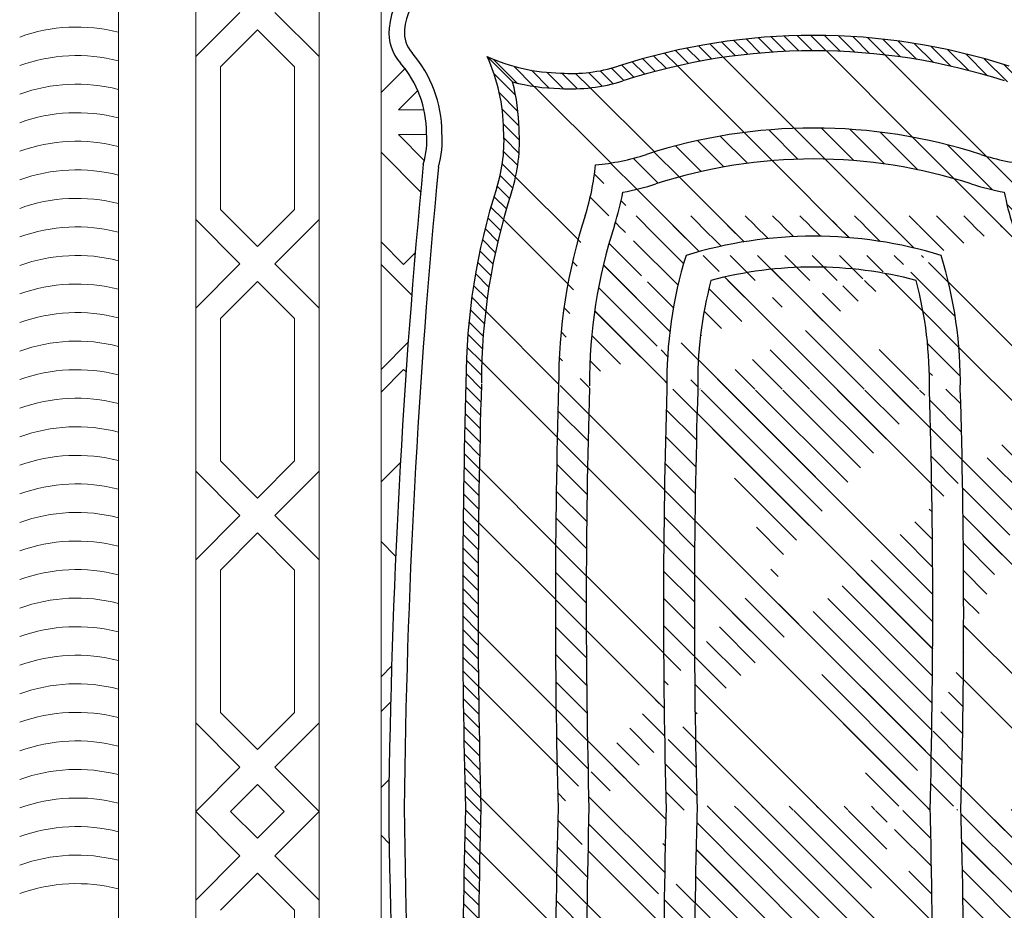
# Model space of a CAD drawing. Units: inches. Extents: x 3592 to 4861, y 1650 to 2243.
# Tile 8 of 30: x 4188.22 to 4207.34, y 1932.29 to 1949.57. Entities that reach past the tile are written whole.
import ezdxf

# ---------------------------------------------------------------- set-up
doc = ezdxf.new("R2010")
doc.units = ezdxf.units.IN
doc.layers.add('A-FURN', color=9, linetype='Continuous', lineweight=13)
doc.layers.add('RA-AP-01$0$INT', color=35, linetype='Continuous', lineweight=5)
for name, color, linetype in [('RA-AP-01$0$FURN', 3, 'Continuous'), ('RA-AP-01$0$WOOD', 64, 'Continuous'), ('RA-AP-02$0$FLPT', 30, 'Continuous')]:
    doc.layers.add(name, color=color, linetype=linetype)

# ---------------------------------------------------------------- blocks, each defined once
blk = doc.blocks.new('A$C67D63ADA')
at = {"layer": 'RA-AP-01$0$INT'}
for p, q in [((4.423181125509104, -6.89561531533655), (4.423181125509032, -6.912102561826093)), ((4.43918112550911, -6.893970246191535), (4.439181125509032, -6.912102561826071)), ((4.439181125509032, -6.912102561826071), (4.455879744655667, -6.89540394267944)), ((4.423181125509032, -6.912102561826093), (4.410714462739163, -6.899635899056222)), ((4.45049483400792, -6.923416270325152), (4.476136761728802, -6.897774342604276)), ((4.515810631825746, -6.901300610639258), (4.523298874513885, -6.908788853327399)), ((4.411867417009952, -6.923416270324986), (4.396098836558103, -6.907647689873135)), ((4.508671457515881, -6.923416270325402), (4.523298874513887, -6.908788853327399)), ((4.543172726542809, -6.903542418296127), (4.523298874513629, -6.923416270325749)), ((4.573619638989622, -6.905854783807836), (4.591181125507156, -6.923416270325372)), ((4.592759678002034, -6.907210300832407), (4.591181125507033, -6.908788853327405)), ((4.591181125507033, -6.908788853327405), (4.605808542505001, -6.923416270325372)), ((4.605808542505038, -6.923416270325409), (4.591181125507032, -6.908788853327405)), ((4.663985166013, -6.923416270325169), (4.651465045800739, -6.910896150112908)), ((4.702612583010966, -6.92341627032501), (4.712072573463438, -6.913956279872539)), ((4.790044040513182, -6.923416270324652), (4.783212045278532, -6.916584275090002)), ((4.806473209230177, -6.917218022043679), (4.812671457513205, -6.923416270326709)), ((4.856598418240554, -6.918206146064184), (4.861808542503289, -6.923416270326919)), ((4.897949975540099, -6.918137752297184), (4.892671457510363, -6.923416270326919)), ((4.877240000006827, -6.923416270326986), (4.277240000006364, -6.923416270324413)), ((4.508671457515881, -6.923416270325401), (4.45049483400792, -6.923416270325152)), ((4.591181125507156, -6.923416270325372), (4.523298874513629, -6.923416270325749)), ((4.605808542505038, -6.923416270325408), (4.663985166013, -6.923416270325169)), ((4.702612583010965, -6.923416270325013), (4.790044040513182, -6.923416270324652)), ((4.877240000006825, -6.923416270326986), (5.477240000007288, -6.923416270324413)), ((4.388754718631812, -6.963416270321417), (4.360068427135066, -6.99210256182739)), ((4.49421056275124, -6.963416270301053), (4.522896854257212, -6.992102561797802)), ((4.551583145753959, -6.963416270316853), (4.522896854257213, -6.992102561822827)), ((4.657038989877026, -6.963416270301689), (4.685725281382997, -6.992102561798438)), ((4.714411572888969, -6.963416270301689), (4.685725281382997, -6.992102561798438)), ((4.819867417008399, -6.963416270316511), (4.848553708505145, -6.992102561822482)), ((4.848553708505147, -6.992102561822486), (4.877240000011487, -6.963416270325371)), ((4.905926291508504, -6.992102561822486), (4.877240000002164, -6.963416270325371)), ((4.934612583005253, -6.963416270316511), (4.905926291508508, -6.992102561822482)), ((4.395382135640173, -6.979416270312523), (4.371382135635868, -7.003416270324554)), ((4.487583145750843, -6.979416270297111), (4.395382135640173, -6.979416270312523)), ((4.487583145750843, -6.979416270297111), (4.511583145760048, -7.003416270298604)), ((4.558210562750208, -6.979416270320077), (4.534210562758016, -7.003416270319991)), ((4.650411572883545, -6.979416270304665), (4.558210562750208, -6.979416270320077)), ((4.650411572883545, -6.979416270304665), (4.674411572885833, -7.00341627029924)), ((4.721038989886534, -6.979416270300584), (4.697038989880161, -7.00341627029924)), ((4.721038989886534, -6.979416270300584), (4.813240000007903, -6.979416270315998)), ((4.813240000007903, -6.979416270315486), (4.837240000004343, -7.003416270319647)), ((4.941240000005749, -6.979416270315486), (4.917240000009309, -7.003416270319647)), ((5.033441010127117, -6.979416270300584), (4.941240000005749, -6.979416270315998)), ((4.859867417002312, -7.003416270323289), (4.877240000006826, -6.986043687324361)), ((4.89461258301134, -7.003416270323289), (4.877240000006826, -6.986043687324361)), ((4.395382135631553, -7.027416270312525), (4.371382135635868, -7.003416270324554)), ((4.48758314576926, -7.027416270297113), (4.511583145760048, -7.003416270298604)), ((4.558210562765816, -7.027416270320077), (4.534210562758016, -7.003416270319991)), ((4.650411572888129, -7.027416270304664), (4.674411572885833, -7.00341627029924)), ((4.721038989873787, -7.027416270300586), (4.697038989880161, -7.00341627029924)), ((4.813240000000789, -7.027416270315487), (4.837240000004343, -7.003416270319647)), ((4.859867417002312, -7.003416270323289), (4.877240000001861, -7.020788853328426)), ((4.89461258301134, -7.003416270323289), (4.877240000011791, -7.020788853328426)), ((4.941240000012863, -7.027416270315487), (4.917240000009309, -7.003416270319647)), ((4.388754718643982, -7.043416270321417), (4.360068427138701, -7.014729978825361)), ((4.494210562764795, -7.043416270301053), (4.52289685426085, -7.01472997879577)), ((4.551583145766129, -7.043416270316853), (4.522896854260848, -7.014729978820797)), ((4.657038989890581, -7.043416270301689), (4.685725281386635, -7.014729978796407)), ((4.714411572875414, -7.043416270301689), (4.685725281379359, -7.014729978796407)), ((4.819867416996229, -7.04341627031651), (4.848553708501509, -7.014729978820453)), ((4.848553708501509, -7.014729978820453), (4.877239999998625, -7.043416270326798)), ((4.905926291512142, -7.014729978820453), (4.877240000015027, -7.043416270326798)), ((4.934612583017423, -7.04341627031651), (4.905926291512142, -7.014729978820453)), ((4.48758314576926, -7.027416270297113), (4.395382135631553, -7.027416270312525)), ((4.650411572888129, -7.027416270304664), (4.558210562765816, -7.027416270320077)), ((4.721038989873787, -7.027416270300586), (4.813239999999876, -7.027416270315999))]:
    blk.add_line(p, q, dxfattribs=at)
for points in [[(5.647240000006826, -6.243416270325369), (5.647240000006826, -7.09341627032537), (4.107240000006826, -7.093416270325372), (4.107240000006826, -6.19341627032537), (4.877240000006826, -6.19341627032537)], [(4.877240000006826, -6.19341627032537), (5.647240000006826, -6.19341627032537), (5.647240000006826, -7.09341627032537), (4.877240000006826, -7.09341627032537)], [(5.597240000006826, -6.243416270325369), (5.597240000006826, -7.04341627032537), (4.157240000006826, -7.043416270325372), (4.157240000006826, -6.243416270325369)], [(4.877240000006826, -6.32341627032537), (4.237240000006825, -6.32341627032537), (4.237240000006825, -6.963416270325371), (4.877240000006826, -6.963416270325371)], [(4.877240000006826, -6.32341627032537), (5.517240000006826, -6.32341627032537), (5.517240000006826, -6.963416270325371), (4.877240000006826, -6.963416270325371)]]:
    blk.add_lwpolyline(points, dxfattribs=at)
for centre, start in [((4.4787219589605, -7.120376270324156), 165.6974573648693), ((4.497201958964411, -7.120376270325429), 165.6974573641792), ((4.515681958963228, -7.120376270326884), 165.697457363391), ((4.534161958959862, -7.12037627032452), 165.697457364672), ((4.552641958963591, -7.120376270324702), 165.6974573645733), ((4.571121958962589, -7.120376270325975), 165.6974573638838), ((4.589601958963954, -7.120376270327248), 165.6974573631937), ((4.608081958962952, -7.120376270325065), 165.6974573643761), ((4.626561958964317, -7.120376270325248), 165.6974573642769), ((4.626561958963465, -7.120376270327612), 165.6974573629959), ((4.645041958962464, -7.120376270325429), 165.6974573641788), ((4.663521958961464, -7.120376270325429), 165.6974573641788), ((4.682001958965192, -7.120376270326703), 165.6974573634886), ((4.700481958964191, -7.120376270325794), 165.6974573639815), ((4.718961958960644, -7.120376270325794), 165.6974573639815), ((4.737441958964554, -7.120376270327067), 165.6974573632914), ((4.755921958963371, -7.120376270328522), 165.6974573625031), ((4.774401958960006, -7.120376270326158), 165.6974573637841), ((4.792881958963734, -7.120376270326339), 165.697457363686), ((4.811361958962733, -7.120376270327612), 165.6974573629959), ((4.829841958964097, -7.120376270328886), 165.6974573623059), ((4.848321958963096, -7.120376270326703), 165.6974573634886), ((4.86680195896446, -7.120376270326884), 165.6974573633905), ((4.885281958960913, -7.120376270329249), 165.6974573621089), ((4.903761958964823, -7.120376270329431), 165.6974573620104), ((4.92224195896364, -7.120376270327067), 165.6974573632914), ((4.940721958962639, -7.12037627032834), 165.6974573626018), ((4.959201958964003, -7.120376270329796), 165.6974573618131), ((4.977681958963002, -7.120376270329796), 165.6974573618131), ((4.996161958962002, -7.120376270327612), 165.6974573629959), ((5.014641958961001, -7.120376270327612), 165.6974573629959), ((5.033121958964729, -7.120376270328886), 165.6974573623059)]:
    blk.add_arc(centre, 0.1091312342836184, start, 199.7961568705686, dxfattribs=at)
blk = doc.blocks.new('A$C09A87C41')
at = {"layer": 'RA-AP-01$0$WOOD'}
h = blk.add_hatch(dxfattribs=at)
h.set_pattern_fill('ANSI31', color=256, scale=0.05, style=0)
h.set_pattern_definition([(45, (0.7182879904584168, -11.54818755465011), (0.0044194173824159, -0.0044194173824159), [])])
edge = h.paths.add_edge_path()
edge.add_ellipse((5.006516613079209, -11.27459283286495), major_axis=(3.435359877543153, 3.435359877543153), ratio=0.9999999999999982, start_angle=403.3022422558093, end_angle=406.5486575131389, ccw=False)
edge.add_ellipse((5.150455045735207, -6.828790194879051), major_axis=(-0.2901946312779826, 0.2901946312779826), ratio=0.9999999999999875, start_angle=297.2093186994243, end_angle=314.9999999999731, ccw=False)
edge.add_ellipse((5.307117976013378, -6.343033378039902), major_axis=(-0.0707106781186454, 0.0707106781186455), ratio=0.9999999999999651, start_angle=116.7779839927149, end_angle=139.0873288843009)
edge.add_ellipse((5.312718414970339, -6.324818905441738), major_axis=(0.0834173982641243, 0.0834173982641243), ratio=0.9999999999999847, start_angle=225.741775187377, end_angle=249.5633269497028)
edge.add_line((5.361758401537698, -6.432112914518591), (5.345299417747169, -6.448571898309089))
edge.add_ellipse((5.312718414970311, -6.32481890544173), major_axis=(-0.0904884660759946, 0.0904884660759945), ratio=0.9999999999999644, start_angle=135.8720682536374, end_angle=149.7498089726665, ccw=False)
edge.add_ellipse((5.307117976013483, -6.343033378039922), major_axis=(-0.0777817459304867, 0.0777817459304867), ratio=0.9999999999999941, start_angle=117.45144083316339, end_angle=138.9346900893823, ccw=False)
edge.add_ellipse((5.150455045735208, -6.82879019487905), major_axis=(0.2831235634661059, 0.2831235634661059), ratio=0.9999999999999859, start_angle=27.03507540014952, end_angle=44.9867285887044)
edge.add_ellipse((5.006516315412802, -11.27459997798134), major_axis=(-3.428298916554014, 3.428298916554014), ratio=0.9999999999999971, start_angle=-46.70235550375367, end_angle=-43.44815559494434)
edge.add_ellipse((4.743915471599394, -11.2745999779814), major_axis=(3.428298916553931, 3.42829891655393), ratio=0.9999999999999994, start_angle=43.44815559494427, end_angle=46.70235550375375)
edge.add_ellipse((4.599976741276995, -6.828790194879051), major_axis=(0.2831235634661173, 0.2831235634661172), ratio=0.9999999999999861, start_angle=45.01327141129749, end_angle=62.96492459984043)
edge.add_ellipse((4.443313810998718, -6.343033378039922), major_axis=(0.0777817459304893, 0.0777817459304893), ratio=0.9999999999999873, start_angle=221.0653099106178, end_angle=242.54855916687399, ccw=False)
edge.add_ellipse((4.437713372041892, -6.32481890544173), major_axis=(0.0904884660759951, 0.0904884660759951), ratio=0.9999999999999603, start_angle=210.2501910273332, end_angle=224.1279317463614, ccw=False)
edge.add_line((4.405132369265034, -6.448571898309089), (4.388673385474508, -6.432112914518594))
edge.add_ellipse((4.43771337204186, -6.324818905441737), major_axis=(0.0834173982641232, 0.0834173982641232), ratio=0.9999999999999797, start_angle=200.4366730503009, end_angle=224.2582248126243)
edge.add_ellipse((4.443313810998827, -6.343033378039902), major_axis=(-0.0707106781186382, 0.0707106781186382), ratio=0.9999999999999952, start_angle=130.9126711156974, end_angle=153.2220160072772)
edge.add_ellipse((4.599976741276995, -6.828790194879051), major_axis=(-0.2901946312779718, 0.2901946312779718), ratio=0.9999999999999895, start_angle=315.0000000000233, end_angle=332.7906813005773, ccw=False)
edge.add_ellipse((4.743915173933024, -11.27459283286497), major_axis=(-3.435359877543123, 3.435359877543123), ratio=0.9999999999999991, start_angle=313.451342486861, end_angle=316.69775774419077, ccw=False)
edge = h.paths.add_edge_path()
edge.add_ellipse((4.299593848995801, -6.48675334004306), major_axis=(-0.0707106781186556, 0.0707106781186556), ratio=0.9999999999999859, start_angle=206.7779839906583, end_angle=229.0873288838364)
edge.add_ellipse((4.281379376397651, -6.481152901086075), major_axis=(-0.0834173982641623, 0.0834173982641623), ratio=0.9999999999999754, start_angle=225.7417751869729, end_angle=249.5633269497573)
edge.add_line((4.388673385474506, -6.432112914518592), (4.405132369265034, -6.448571898309089))
edge.add_ellipse((4.281379376397657, -6.481152901086004), major_axis=(-0.0904884660760182, 0.0904884660760182), ratio=0.9999999999999957, start_angle=225.8720682533453, end_angle=239.7498089726896, ccw=False)
edge.add_ellipse((4.299593848995796, -6.486753340043026), major_axis=(0.0777817459305317, 0.0777817459305317), ratio=0.9999999999999891, start_angle=297.4514408381613, end_angle=318.9346900891407, ccw=False)
edge.add_ellipse((4.785350665835052, -6.643416270320893), major_axis=(0.2831235634661102, 0.2831235634661102), ratio=0.9999999999999978, start_angle=117.0350753988375, end_angle=152.9649246009711)
edge.add_ellipse((4.299593848995777, -6.800079200598784), major_axis=(-0.0777817459305426, 0.0777817459305426), ratio=0.9999999999999973, start_angle=221.0653099111909, end_angle=242.5485591625442, ccw=False)
edge.add_ellipse((4.281379376397679, -6.805679639555494), major_axis=(-0.0904884660760244, 0.0904884660760244), ratio=0.9999999999999076, start_angle=210.2501910270576, end_angle=224.1279317467988, ccw=False)
edge.add_line((4.405132369264926, -6.838260642332959), (4.388673385474263, -6.854719626123697))
edge.add_ellipse((4.281379376397679, -6.80567963955562), major_axis=(0.0834173982641642, 0.0834173982641642), ratio=0.9999999999999609, start_angle=290.4366730499258, end_angle=314.2582248131156)
edge.add_ellipse((4.299593848995804, -6.800079200598786), major_axis=(-0.0707106781186612, 0.0707106781186612), ratio=0.999999999999977, start_angle=220.9126711163551, end_angle=243.222016008517)
edge.add_ellipse((4.785350665835053, -6.643416270320894), major_axis=(0.2901946312779783, 0.2901946312779783), ratio=0.9999999999999984, start_angle=117.2093186999746, end_angle=152.7906813002342, ccw=False)
edge = h.paths.add_edge_path()
edge.add_ellipse((4.743915471599392, -2.012232562660299), major_axis=(3.428298916553894, 3.428298916553894), ratio=0.9999999999999992, start_angle=223.2976444962459, end_angle=226.5518444050561)
edge.add_ellipse((5.006516315412771, -2.012232562660296), major_axis=(3.428298916553752, 3.428298916553752), ratio=0.9999999999999971, start_angle=223.448155594945, end_angle=226.7023555037531)
edge.add_ellipse((5.150455045735209, -6.458042345762599), major_axis=(0.283123563466111, 0.283123563466111), ratio=0.999999999999996, start_angle=225.0132714112834, end_angle=242.9649246011241)
edge.add_ellipse((5.30711797601273, -6.94379916260194), major_axis=(0.0777817459305174, 0.0777817459305174), ratio=0.9999999999999873, start_angle=401.06530991071423, end_angle=422.548559161793, ccw=False)
edge.add_ellipse((5.312718414969516, -6.962013635200094), major_axis=(0.0904884660760023, 0.0904884660760023), ratio=0.9999999999999566, start_angle=390.2501910269164, end_angle=404.12793174642553, ccw=False)
edge.add_line((5.345299417747278, -6.838260642332959), (5.361758401537942, -6.854719626123698))
edge.add_ellipse((5.312718414969516, -6.962013635200098), major_axis=(0.0834173982641439, 0.0834173982641439), ratio=0.9999999999999785, start_angle=20.43667304973462, end_angle=44.25822481258737)
edge.add_ellipse((5.307117976012772, -6.943799162601948), major_axis=(-0.0707106781186618, 0.0707106781186618), ratio=0.999999999999977, start_angle=-49.08732888421749, end_angle=-26.77798399064677)
edge.add_ellipse((5.150455045735209, -6.458042345762597), major_axis=(0.2901946312779783, 0.2901946312779783), ratio=0.9999999999999957, start_angle=225.0000000000273, end_angle=242.7906812999824, ccw=False)
edge.add_ellipse((5.006516613079198, -2.012239707776725), major_axis=(3.43535987754352, 3.43535987754352), ratio=0.999999999999996, start_angle=223.4513424868609, end_angle=226.697757744191, ccw=False)
edge.add_ellipse((4.743915173933023, -2.012239707776712), major_axis=(3.435359877543229, 3.435359877543229), ratio=0.9999999999999998, start_angle=223.3022422558095, end_angle=226.5486575131387, ccw=False)
edge.add_ellipse((4.599976741276995, -6.458042345762597), major_axis=(0.2901946312779746, 0.2901946312779748), ratio=0.9999999999999964, start_angle=207.2093187000184, end_angle=224.9999999999795, ccw=False)
edge.add_ellipse((4.443313810999427, -6.943799162601947), major_axis=(-0.070710678118668, 0.070710678118668), ratio=0.9999999999999838, start_angle=-63.22201600935903, end_angle=-40.9126711157662)
edge.add_ellipse((4.437713372042683, -6.962013635200099), major_axis=(0.0834173982641484, 0.0834173982641484), ratio=0.9999999999999729, start_angle=45.74177518742643, end_angle=69.56332695026246)
edge.add_line((4.388673385474263, -6.854719626123697), (4.405132369264926, -6.838260642332958))
edge.add_ellipse((4.437713372042681, -6.962013635200094), major_axis=(0.0904884660760224, 0.0904884660760225), ratio=0.9999999999999282, start_angle=405.87206825357924, end_angle=419.7498089730807, ccw=False)
edge.add_ellipse((4.443313810999475, -6.94379916260194), major_axis=(-0.0777817459305165, 0.0777817459305165), ratio=0.9999999999999927, start_angle=297.4514408382556, end_angle=318.93469008929503, ccw=False)
edge.add_ellipse((4.599976741276995, -6.458042345762597), major_axis=(0.2831235634661077, 0.2831235634661077), ratio=0.9999999999999937, start_angle=207.0350753988627, end_angle=224.9867285886981)
edge = h.paths.add_edge_path()
edge.add_ellipse((5.450837938016399, -6.800079200598789), major_axis=(-0.0707106781186565, 0.0707106781186565), ratio=0.9999999999999875, start_angle=26.77798399147072, end_angle=49.08732888364846)
edge.add_ellipse((5.469052410614524, -6.80567963955562), major_axis=(0.0834173982641601, 0.0834173982641601), ratio=0.9999999999999984, start_angle=135.7417751868887, end_angle=159.563326950074)
edge.add_line((5.36175840153794, -6.854719626123697), (5.345299417747278, -6.838260642332959))
edge.add_ellipse((5.469052410614523, -6.805679639555488), major_axis=(0.0904884660760307, 0.0904884660760307), ratio=0.9999999999999984, start_angle=135.8720682531977, end_angle=149.7498089729454, ccw=False)
edge.add_ellipse((5.450837938016426, -6.800079200598787), major_axis=(0.0777817459305426, 0.0777817459305427), ratio=0.9999999999999968, start_angle=117.4514408374904, end_angle=138.9346900888003, ccw=False)
edge.add_ellipse((4.965081121177151, -6.643416270320895), major_axis=(-0.2831235634661119, 0.2831235634661119), ratio=0.9999999999999992, start_angle=207.0350753990193, end_angle=242.9649246011595)
edge.add_ellipse((5.450837938016407, -6.486753340043026), major_axis=(0.0777817459305285, 0.0777817459305285), ratio=0.9999999999999747, start_angle=131.0653099108597, end_angle=152.5485591618505, ccw=False)
edge.add_ellipse((5.469052410614547, -6.481152901086004), major_axis=(0.09048846607603, 0.09048846607603), ratio=0.9999999999999619, start_angle=120.25019102731059, end_angle=134.1279317466551, ccw=False)
edge.add_line((5.345299417747169, -6.448571898309089), (5.361758401537697, -6.432112914518592))
edge.add_ellipse((5.469052410614551, -6.481152901086075), major_axis=(-0.0834173982641603, 0.0834173982641603), ratio=0.9999999999999998, start_angle=20.43667305024269, end_angle=44.25822481302925)
edge.add_ellipse((5.450837938016403, -6.486753340043062), major_axis=(-0.0707106781186603, 0.0707106781186603), ratio=0.9999999999999737, start_angle=40.91267111616517, end_angle=63.22201600943157)
edge.add_ellipse((4.965081121177149, -6.643416270320895), major_axis=(0.2901946312779771, 0.2901946312779771), ratio=0.9999999999999992, start_angle=297.2093186997686, end_angle=332.7906813000034, ccw=False)
h = blk.add_hatch(dxfattribs=at)
h.set_pattern_fill('ANSI32', color=256, scale=0.2, style=0)
h.set_pattern_definition([(45, (0.7182879904584168, -11.54818755465011), (0.0530330085889911, -0.0530330085889911), []), (45, (0.7182879904584168, -11.51283221565011), (0.0530330085889911, -0.0530330085889911), [])])
edge = h.paths.add_edge_path()
edge.add_ellipse((5.15045504573521, -6.82879019487905), major_axis=(-0.2831235634661157, 0.2831235634661156), ratio=0.9999999999999889, start_angle=297.21454354460053, end_angle=314.98672858870884, ccw=False)
edge.add_ellipse((5.307117976013485, -6.343033378039922), major_axis=(-0.0777817459304881, 0.0777817459304881), ratio=0.9999999999999928, start_angle=116.7981781115797, end_angle=138.9346900893818)
edge.add_ellipse((5.312718414970311, -6.32481890544173), major_axis=(-0.0904884660759946, 0.0904884660759946), ratio=0.9999999999999658, start_angle=135.8720682536378, end_angle=149.7498089726664)
edge.add_ellipse((5.469052410614547, -6.481152901086004), major_axis=(0.0904884660760303, 0.0904884660760302), ratio=0.9999999999999603, start_angle=120.2501910273106, end_angle=134.1279317466551)
edge.add_ellipse((5.450837938016407, -6.486753340043026), major_axis=(-0.0777817459305327, 0.0777817459305327), ratio=0.9999999999999915, start_angle=41.06530991085969, end_angle=63.20182189333976)
edge.add_ellipse((4.965081121177151, -6.643416270320894), major_axis=(-0.2831235634661133, 0.2831235634661133), ratio=0.9999999999999984, start_angle=207.214543545815, end_angle=242.7854564539869, ccw=False)
edge.add_ellipse((5.450837938016426, -6.800079200598786), major_axis=(0.0777817459305424, 0.0777817459305424), ratio=0.9999999999999962, start_angle=116.7981781073729, end_angle=138.9346900888086)
edge.add_ellipse((5.469052410614524, -6.805679639555493), major_axis=(0.0904884660760289, 0.0904884660760289), ratio=0.9999999999999841, start_angle=135.872068253202, end_angle=149.7498089729424)
edge.add_ellipse((5.312718414969522, -6.962013635200094), major_axis=(-0.0904884660760224, 0.0904884660760225), ratio=0.9999999999999282, start_angle=-59.7498089730807, end_angle=-45.87206825357926)
edge.add_ellipse((5.307117976012728, -6.94379916260194), major_axis=(0.0777817459305181, 0.0777817459305181), ratio=0.9999999999999861, start_angle=41.06530991070497, end_angle=63.20182189334603)
edge.add_ellipse((5.150455045735208, -6.458042345762599), major_axis=(0.2831235634661146, 0.2831235634661146), ratio=0.9999999999999907, start_angle=225.013271411291, end_angle=242.7854564539341, ccw=False)
edge.add_ellipse((5.006516315412806, -2.012232562660296), major_axis=(3.428298916554143, 3.428298916554143), ratio=0.9999999999999941, start_angle=223.4481555949448, end_angle=226.7023555037533, ccw=False)
edge.add_ellipse((4.743915471599424, -2.012232562660299), major_axis=(3.428298916554168, 3.428298916554171), ratio=0.9999999999999991, start_angle=223.2976444962462, end_angle=226.551844405056, ccw=False)
edge.add_ellipse((4.599976741276996, -6.458042345762597), major_axis=(0.2831235634661098, 0.2831235634661098), ratio=0.9999999999999973, start_angle=207.2145435460398, end_angle=224.9867285887048, ccw=False)
edge.add_ellipse((4.443313810999473, -6.94379916260194), major_axis=(-0.0777817459305183, 0.0777817459305183), ratio=0.9999999999999823, start_angle=-63.2018218932521, end_angle=-41.06530991071377)
edge.add_ellipse((4.437713372042686, -6.962013635200094), major_axis=(-0.0904884660760028, 0.0904884660760028), ratio=0.9999999999999504, start_angle=-44.12793174642511, end_angle=-30.25019102691602)
edge.add_ellipse((4.281379376397679, -6.80567963955549), major_axis=(-0.0904884660760215, 0.0904884660760215), ratio=0.9999999999999245, start_angle=210.2501910270558, end_angle=224.1279317467963)
edge.add_ellipse((4.299593848995777, -6.800079200598786), major_axis=(0.077781745930539, 0.077781745930539), ratio=0.999999999999963, start_angle=311.0653099111909, end_angle=333.2018218926339)
edge.add_ellipse((4.785350665835052, -6.643416270320894), major_axis=(0.2831235634661089, 0.2831235634661091), ratio=0.9999999999999989, start_angle=117.21454354600829, end_angle=152.7854564541833, ccw=False)
edge.add_ellipse((4.299593848995796, -6.486753340043026), major_axis=(0.077781745930533, 0.077781745930533), ratio=0.9999999999999792, start_angle=296.7981781066777, end_angle=318.9346900891398)
edge.add_ellipse((4.281379376397657, -6.481152901086003), major_axis=(-0.0904884660760217, 0.0904884660760217), ratio=0.9999999999999742, start_angle=225.872068253344, end_angle=239.7498089726891)
edge.add_ellipse((4.437713372041892, -6.32481890544173), major_axis=(0.090488466075997, 0.090488466075997), ratio=0.9999999999999756, start_angle=210.2501910273331, end_angle=224.1279317463622)
edge.add_ellipse((4.44331381099872, -6.343033378039923), major_axis=(0.0777817459304873, 0.0777817459304872), ratio=0.9999999999999861, start_angle=221.0653099106177, end_angle=243.2018218883976)
edge.add_ellipse((4.599976741276995, -6.828790194879051), major_axis=(-0.2831235634661067, 0.2831235634661067), ratio=0.9999999999999895, start_angle=315.01327141129775, end_angle=332.78545645540567, ccw=False)
edge.add_ellipse((4.743915471599392, -11.2745999779814), major_axis=(-3.428298916553902, 3.428298916553902), ratio=0.9999999999999984, start_angle=313.4481555949443, end_angle=316.7023555037538, ccw=False)
edge.add_ellipse((5.006516315412786, -11.27459997798134), major_axis=(-3.428298916554052, 3.428298916554052), ratio=1, start_angle=313.29764449624645, end_angle=316.5518444050555, ccw=False)
edge = h.paths.add_edge_path(flags=16)
edge.add_ellipse((4.745320840887742, -11.27459782170807), major_axis=(3.392940520945516, 3.392940520945516), ratio=1, start_angle=43.44876692339471, end_angle=46.71249975461917)
edge.add_ellipse((4.599976741276995, -6.828790194878992), major_axis=(-0.2477682244067734, 0.2477682244067734), ratio=0.9999999999999911, start_angle=-45.31868720933983, end_angle=-27.00912183057358)
edge.add_ellipse((4.443313810998828, -6.343033378039872), major_axis=(0.1131370849898469, 0.1131370849898469), ratio=0.9999999999999724, start_angle=230.5682590208478, end_angle=242.6218359751805, ccw=False)
edge.add_ellipse((4.299593848995757, -6.486753340043112), major_axis=(-0.1131370849898624, 0.1131370849898624), ratio=0.9999999999999953, start_angle=207.3781640250758, end_angle=219.4317409792351, ccw=False)
edge.add_ellipse((4.78535066583505, -6.643416270320884), major_axis=(0.2477682244067863, 0.2477682244067863), ratio=0.9999999999999974, start_angle=117.0091218305267, end_angle=152.9908781690427)
edge.add_ellipse((4.299593848995773, -6.800079200598856), major_axis=(0.1131370849898833, 0.1131370849898833), ratio=0.9999999999999682, start_angle=320.56825902084296, end_angle=332.62183597593753, ccw=False)
edge.add_ellipse((4.443313810999473, -6.943799162601939), major_axis=(0.1131370849898351, 0.1131370849898351), ratio=0.9999999999999213, start_angle=387.3781640246361, end_angle=399.43174097937606, ccw=False)
edge.add_ellipse((4.599976741276996, -6.458042345762606), major_axis=(0.2477682244067743, 0.2477682244067742), ratio=0.99999999999999, start_angle=207.0091218307682, end_angle=225.3186872093523)
edge.add_ellipse((4.745320840887777, -2.012234718933553), major_axis=(-3.392940520945741, 3.392940520945741), ratio=0.9999999999999992, start_angle=133.2875002453813, end_angle=136.5512330766047)
edge.add_ellipse((5.005110946124445, -2.012234718933546), major_axis=(3.392940520945412, 3.392940520945411), ratio=0.9999999999999989, start_angle=223.4487669233947, end_angle=226.7124997546191)
edge.add_ellipse((5.150455045735207, -6.458042345762608), major_axis=(-0.2477682244067739, 0.2477682244067739), ratio=0.9999999999999966, start_angle=134.6813127906568, end_angle=152.9908781692236)
edge.add_ellipse((5.30711797601273, -6.943799162601939), major_axis=(-0.1131370849898406, 0.1131370849898406), ratio=0.9999999999999811, start_angle=320.568259020624, end_angle=332.62183597538194, ccw=False)
edge.add_ellipse((5.45083793801643, -6.800079200598855), major_axis=(0.113137084989895, 0.113137084989895), ratio=0.999999999999955, start_angle=117.3781640240419, end_angle=129.4317409791577, ccw=False)
edge.add_ellipse((4.965081121177152, -6.643416270320884), major_axis=(0.2477682244067847, 0.2477682244067847), ratio=0.9999999999999992, start_angle=297.0091218309669, end_angle=332.990878169475)
edge.add_ellipse((5.450837938016447, -6.486753340043118), major_axis=(-0.1131370849898789, 0.1131370849898789), ratio=0.9999999999999342, start_angle=50.56825902076281, end_angle=62.62183597491821, ccw=False)
edge.add_ellipse((5.30711797601337, -6.34303337803987), major_axis=(0.1131370849898374, 0.1131370849898374), ratio=0.9999999999999493, start_angle=207.3781640247929, end_angle=219.4317409791543, ccw=False)
edge.add_ellipse((5.150455045735204, -6.828790194878992), major_axis=(-0.2477682244067807, 0.2477682244067808), ratio=0.9999999999999934, start_angle=-62.99087816941401, end_angle=-44.68131279065508)
edge.add_ellipse((5.005110946124442, -11.27459782170805), major_axis=(3.392940520945543, 3.392940520945543), ratio=0.9999999999999974, start_angle=43.28750024538099, end_angle=46.55123307660507)
edge = h.paths.add_edge_path(flags=0)
edge.add_ellipse((4.745321446260899, -11.27461227828643), major_axis=(3.378818834290158, 3.378818834290157), ratio=0.9999999999999996, start_angle=43.44228925150885, end_angle=46.72161971502517)
edge.add_ellipse((4.599976741276998, -6.828790194878991), major_axis=(-0.2336260887830454, 0.2336260887830454), ratio=0.9999999999999974, start_angle=-45.30974264369766, end_angle=-26.99844483641433)
edge.add_ellipse((4.443313810998811, -6.343033378039858), major_axis=(0.1272792206135962, 0.1272792206135962), ratio=0.9999999999999403, start_angle=235.6264990356023, end_angle=242.6432427499436, ccw=False)
edge.add_ellipse((4.299593848995773, -6.486753340043007), major_axis=(0.1272792206136285, 0.1272792206136286), ratio=0.9999999999999204, start_angle=297.35675724967757, end_angle=304.3735009644582, ccw=False)
edge.add_ellipse((4.785350665835048, -6.643416270320905), major_axis=(0.2336260887830504, 0.2336260887830504), ratio=0.9999999999999921, start_angle=116.998444836676, end_angle=153.0015551636886)
edge.add_ellipse((4.299593848995741, -6.800079200598703), major_axis=(-0.1272792206136906, 0.1272792206136906), ratio=0.9999999999996289, start_angle=235.62649903554922, end_angle=242.64324274961962, ccw=False)
edge.add_ellipse((4.443313810999469, -6.943799162601998), major_axis=(-0.1272792206136219, 0.1272792206136219), ratio=0.9999999999999658, start_angle=297.3567572500489, end_angle=304.3735009646209, ccw=False)
edge.add_ellipse((4.599976741276995, -6.458042345762605), major_axis=(0.2336260887830445, 0.2336260887830445), ratio=0.9999999999999957, start_angle=206.9984448365414, end_angle=225.3097426436968)
edge.add_ellipse((4.745321446260921, -2.012220262355212), major_axis=(3.378818834290089, 3.378818834290088), ratio=0.9999999999999994, start_angle=223.2783802849744, end_angle=226.5577107484907)
edge.add_ellipse((5.005110340751275, -2.012220262355198), major_axis=(3.378818834290274, 3.378818834290274), ratio=0.9999999999999992, start_angle=223.4422892515091, end_angle=226.7216197150253)
edge.add_ellipse((5.150455045735206, -6.458042345762609), major_axis=(0.2336260887830463, 0.2336260887830463), ratio=0.9999999999999937, start_angle=224.6902573562994, end_angle=243.0015551634542)
edge.add_ellipse((5.30711797601273, -6.943799162602), major_axis=(-0.1272792206135949, 0.1272792206135949), ratio=0.9999999999997138, start_angle=325.62649903537766, end_angle=332.6432427499585, ccw=False)
edge.add_ellipse((5.450837938016461, -6.800079200598699), major_axis=(-0.1272792206135936, 0.1272792206135936), ratio=0.999999999999666, start_angle=27.356757250387716, end_angle=34.37350096445232, ccw=False)
edge.add_ellipse((4.965081121177155, -6.643416270320904), major_axis=(0.23362608878305, 0.23362608878305), ratio=0.9999999999999992, start_angle=296.9984448363078, end_angle=333.0015551633219)
edge.add_ellipse((5.450837938016428, -6.486753340043003), major_axis=(0.1272792206136045, 0.1272792206136045), ratio=0.9999999999999529, start_angle=145.6264990355431, end_angle=152.6432427503271, ccw=False)
edge.add_ellipse((5.307117976013396, -6.34303337803986), major_axis=(0.1272792206135615, 0.1272792206135615), ratio=0.9999999999996925, start_angle=207.3567572500474, end_angle=214.3735009643965, ccw=False)
edge.add_ellipse((5.150455045735208, -6.828790194878991), major_axis=(-0.2336260887830484, 0.2336260887830485), ratio=0.9999999999999953, start_angle=-63.00155516358085, end_angle=-44.69025735630093)
edge.add_ellipse((5.005110340751286, -11.27461227828636), major_axis=(-3.378818834290266, 3.378818834290266), ratio=0.9999999999999998, start_angle=-46.72161971502535, end_angle=-43.44228925150914)
edge = h.paths.add_edge_path(flags=0)
edge.add_ellipse((4.747128261062206, -11.27459926241731), major_axis=(-3.343445075648777, 3.343445075648777), ratio=0.9999999999999991, start_angle=-46.55229325491085, end_angle=-43.26504392007965)
edge.add_ellipse((4.599976741277094, -6.828790194878977), major_axis=(0.198270749723715, 0.198270749723715), ratio=0.999999999999988, start_angle=44.18347671010175, end_angle=62.12936993332099)
edge.add_ellipse((4.785350665835048, -6.643416270320889), major_axis=(0.198270749723727, 0.198270749723727), ratio=0.9999999999999971, start_angle=117.8706300667295, end_angle=152.1293699332338)
edge.add_ellipse((4.599976741276998, -6.458042345762598), major_axis=(0.1982707497237202, 0.1982707497237202), ratio=0.9999999999999882, start_angle=207.8706300666892, end_angle=225.8165232899116)
edge.add_ellipse((4.747128261062279, -2.01223327822427), major_axis=(-3.343445075648579, 3.34344507564858), ratio=0.9999999999999984, start_angle=133.2650439200784, end_angle=136.5522932549098)
edge.add_ellipse((5.003303525949927, -2.012233278224277), major_axis=(-3.343445075648679, 3.343445075648679), ratio=0.9999999999999996, start_angle=133.4477067450899, end_angle=136.7349560799216)
edge.add_ellipse((5.150455045735204, -6.458042345762598), major_axis=(-0.1982707497237223, 0.1982707497237223), ratio=0.9999999999999994, start_angle=134.1834767100914, end_angle=152.1293699333112)
edge.add_ellipse((4.965081121177155, -6.643416270320892), major_axis=(0.1982707497237268, 0.1982707497237267), ratio=0.9999999999999987, start_angle=297.8706300667671, end_angle=332.1293699332712)
edge.add_ellipse((5.150455045735109, -6.828790194878977), major_axis=(0.1982707497237106, 0.1982707497237105), ratio=0.9999999999999982, start_angle=27.87063006667902, end_angle=45.8165232898948)
edge.add_ellipse((5.00330352595001, -11.2745992624173), major_axis=(3.343445075648743, 3.343445075648743), ratio=0.9999999999999996, start_angle=43.26504392007961, end_angle=46.55229325491089)
edge = h.paths.add_edge_path(flags=0)
edge.add_ellipse((4.747685770081003, -11.27459857725902), major_axis=(3.329301968186143, 3.329301968186141), ratio=0.9999999999999989, start_angle=43.44789769190167, end_angle=46.74269456932172)
edge.add_ellipse((4.599976741277087, -6.828790194878972), major_axis=(-0.1841286140999701, 0.1841286140999702), ratio=0.9999999999999841, start_angle=-45.99531238101485, end_angle=-30.22398030679106)
edge.add_ellipse((4.785350665835029, -6.643416270320906), major_axis=(0.1841286140999794, 0.1841286140999793), ratio=0.9999999999999998, start_angle=120.2239803068321, end_angle=149.7760196931203)
edge.add_ellipse((4.599976741276998, -6.458042345762589), major_axis=(0.1841286140999956, 0.1841286140999956), ratio=0.9999999999999953, start_angle=210.2239803068005, end_angle=225.9953123810239)
edge.add_ellipse((4.747685770081015, -2.012233963382593), major_axis=(-3.329301968186209, 3.32930196818621), ratio=0.9999999999999991, start_angle=133.2573054306775, end_angle=136.5521023080975)
edge.add_ellipse((5.002746016931159, -2.012233963382618), major_axis=(-3.329301968186245, 3.329301968186245), ratio=0.9999999999999984, start_angle=133.447897691902, end_angle=136.7426945693227)
edge.add_ellipse((5.150455045735208, -6.458042345762592), major_axis=(-0.1841286140999912, 0.1841286140999912), ratio=0.9999999999999873, start_angle=134.0046876189747, end_angle=149.7760196931988)
edge.add_ellipse((4.965081121177172, -6.643416270320907), major_axis=(-0.1841286140999788, 0.1841286140999788), ratio=0.9999999999999968, start_angle=210.2239803068796, end_angle=239.7760196931682)
edge.add_ellipse((5.150455045735117, -6.82879019487897), major_axis=(0.1841286140999714, 0.1841286140999713), ratio=0.9999999999999896, start_angle=30.22398030679139, end_angle=45.99531238102014)
edge.add_ellipse((5.002746016931209, -11.274598577259), major_axis=(3.329301968186158, 3.329301968186158), ratio=1, start_angle=43.25730543067866, end_angle=46.5521023080979)
h = blk.add_hatch(dxfattribs=at)
h.set_pattern_fill('ANSI31', color=256, scale=0.1, style=0)
h.set_pattern_definition([(45, (0.7182879904584168, -11.54818755465011), (0.0088388347648318, -0.0088388347648318), [])])
edge = h.paths.add_edge_path(flags=16)
edge.add_arc((4.965081121177173, -6.643416270320907), 0.2603971832811541, 345.2239803068796, 374.7760196931681)
edge.add_arc((4.965081121177173, -6.643416270320907), 0.2603971832811541, -14.776019693120418, 14.77601969316811, ccw=False)
edge = h.paths.add_edge_path(flags=16)
edge.add_arc((4.785350665835029, -6.643416270320907), 0.2603971832811541, 165.223980306832, 194.7760196931204)
edge.add_arc((4.785350665835029, -6.643416270320907), 0.2603971832811541, 165.223980306832, 194.7760196931204, ccw=False)
edge = h.paths.add_edge_path(flags=0)
edge.add_arc((4.785350665835029, -6.643416270320907), 0.2603971832811541, 165.223980306832, 194.7760196931204)
edge.add_arc((4.785350665835029, -6.643416270320907), 0.2603971832811541, 165.223980306832, 194.7760196931204, ccw=False)
edge = h.paths.add_edge_path(flags=0)
edge.add_arc((4.785350665835029, -6.643416270320907), 0.2603971832811541, 165.223980306832, 194.7760196931204)
edge.add_arc((4.785350665835029, -6.643416270320907), 0.2603971832811541, 165.223980306832, 194.7760196931204, ccw=False)
edge = h.paths.add_edge_path(flags=0)
edge.add_arc((4.785350665835029, -6.643416270320907), 0.2603971832811541, 165.223980306832, 194.7760196931204)
edge.add_arc((4.785350665835029, -6.643416270320907), 0.2603971832811541, 165.223980306832, 194.7760196931204, ccw=False)
edge = h.paths.add_edge_path(flags=0)
edge.add_arc((4.785350665835029, -6.643416270320907), 0.2603971832811541, 165.223980306832, 194.7760196931204)
edge.add_arc((4.785350665835029, -6.643416270320907), 0.2603971832811541, 165.223980306832, 194.7760196931204, ccw=False)
edge = h.paths.add_edge_path(flags=0)
edge.add_arc((4.785350665835029, -6.643416270320907), 0.2603971832811541, 165.223980306832, 194.7760196931204)
edge.add_arc((4.785350665835029, -6.643416270320907), 0.2603971832811541, 165.223980306832, 194.7760196931204, ccw=False)
edge = h.paths.add_edge_path(flags=0)
edge.add_arc((4.785350665835029, -6.643416270320907), 0.2603971832811541, 165.223980306832, 194.7760196931204)
edge.add_arc((4.785350665835029, -6.643416270320907), 0.2603971832811541, 165.223980306832, 194.7760196931204, ccw=False)
edge = h.paths.add_edge_path()
edge.add_arc((5.30711797601273, -6.943799162601939), 0.1599999999999918, 95.56825902062381, 107.6218359753744)
edge.add_arc((5.150455045735207, -6.458042345762605), 0.3503971832811637, 269.6813127906517, 287.9908781692269)
edge.add_arc((5.307117976013371, -6.34303337803987), 0.1599999999999917, 252.3781640232651, 264.4317409791539)
edge.add_arc((4.965081121177153, -6.643416270320884), 0.3503971832811761, 342.0091218309644, 377.9908781694648)
edge.add_arc((5.005110946124438, -2.012234718933557), 4.798342501046485, 268.4423197280547, 271.7124997546188)
edge.add_arc((5.150455045735207, -6.828790194878991), 0.3503971832811637, 72.00912183077308, 90.31868720934834)
edge.add_arc((5.005110340751293, -2.012220262355208), 4.778371420254705, 268.433225420277, 271.7034061068158)
edge.add_arc((5.150455045735207, -6.828790194878991), 0.3303971832811637, 72.00912183077308, 90.31868720934834)
edge.add_arc((5.005110340751291, -11.27461227828638), 4.7783714202547, 88.29659389318418, 91.5667745797229)
edge.add_arc((5.450837938016446, -6.486753340043115), 0.1600000000000254, 185.5682590207637, 197.6218359749416)
edge.add_arc((5.450837938016429, -6.800079200598855), 0.1600000000000541, 162.3781640240467, 174.4317409791574)
edge.add_arc((5.307117976012735, -6.943799162601998), 0.1800000000000505, 100.6264990353792, 107.6432427499818)
edge.add_arc((5.307117976013394, -6.343033378039859), 0.1800000000000069, 252.3567572486067, 259.3735009643972)
edge.add_arc((5.45083793801643, -6.486753340043007), 0.1800000000000424, 190.6264990355417, 197.6432427503393)
edge.add_arc((4.965081121177155, -6.643416270320905), 0.3303971832811676, 341.9984448362978, 378.0015551633146)
edge.add_arc((5.450837938016462, -6.800079200598699), 0.1800000000000547, 162.3567572504062, 169.373500964452)
edge.add_arc((5.150455045735206, -6.458042345762599), 0.2803971832811691, 269.1834767100981, 287.1293699333106)
edge.add_arc((5.150455045735107, -6.828790194878977), 0.2803971832811534, 72.87063006667864, 90.81652328989695)
edge.add_arc((4.965081121177155, -6.643416270320891), 0.2803971832811769, 342.8706300667665, 377.1293699332709)
edge.add_arc((5.150455045735205, -6.45804234576259), 0.2603971832811776, 269.0046876189688, 284.7760196931993)
edge.add_arc((5.150455045735117, -6.828790194878972), 0.2603971832811458, 75.22398030679119, 90.99531238102313)
edge.add_arc((5.150455045735207, -6.458042345762605), 0.3303971832811637, 269.6813127906517, 287.9908781692269)
edge.add_arc((5.003303525949946, -2.012233278224274), 4.728345371032053, 268.4320043718199, 271.7349560799219)
edge.add_arc((5.003303525949998, -11.27459926241731), 4.728345371032045, 88.2650439200796, 91.56799562818075)
edge.add_arc((5.00274601693117, -2.012233963382607), 4.708343996644348, 268.4295004240392, 271.7426945693223)
edge.add_arc((5.002746016931202, -11.274598577259), 4.708343996644358, 88.25730543067873, 91.57049957596126)
edge.add_arc((4.747685770080999, -11.274598577259), 4.708343996644359, 88.42950042403872, 91.74269456932127)
edge.add_arc((4.747685770081036, -2.012233963382596), 4.708343996644359, 268.2573054306777, 271.5704995759608)
edge.add_arc((4.747128261062202, -11.27459926241732), 4.728345371032054, 88.43200437181925, 91.73495607992041)
edge.add_arc((4.747128261062259, -2.012233278224274), 4.728345371032054, 268.265043920078, 271.56799562818)
edge.add_arc((4.74532144626091, -11.27461227828638), 4.778371420254699, 88.43322542027705, 91.7034061068158)
edge.add_arc((4.599976741276996, -6.828790194878991), 0.3303971832811637, 89.68131279065165, 107.9908781692269)
edge.add_arc((4.599976741276996, -6.458042345762605), 0.3303971832811637, 252.0091218307731, 270.3186872093484)
edge.add_arc((4.745321446260912, -2.012220262355208), 4.778371420254705, 268.2965938931842, 271.5667745797229)
edge.add_arc((4.599976741276996, -6.828790194878991), 0.3503971832811637, 89.68131279065165, 107.9908781692269)
edge.add_arc((4.745320840887767, -2.012234718933562), 4.79834250104648, 268.2875002453812, 271.5576802719454)
edge.add_arc((4.599976741277086, -6.828790194878972), 0.2603971832811458, 89.00468761897682, 104.7760196932087)
edge.add_arc((4.599976741276998, -6.45804234576259), 0.2603971832811776, 255.2239803068007, 270.9953123810312)
edge.add_arc((4.785350665835048, -6.643416270320891), 0.2803971832811769, 162.8706300667291, 197.1293699332334)
edge.add_arc((4.599976741277096, -6.828790194878977), 0.2803971832811534, 89.183476710103, 107.1293699333213)
edge.add_arc((4.599976741276996, -6.458042345762599), 0.2803971832811691, 252.8706300666894, 270.816523289902)
edge.add_arc((4.299593848995741, -6.800079200598699), 0.1800000000000547, 10.626499035548, 17.64324274959381)
edge.add_arc((4.785350665835048, -6.643416270320905), 0.3303971832811676, 161.9984448366853, 198.0015551637021)
edge.add_arc((4.299593848995773, -6.486753340043007), 0.1800000000000424, 342.3567572496606, 349.3735009644582)
edge.add_arc((4.44331381099881, -6.343033378039859), 0.1800000000000069, 280.6264990356027, 287.6432427513933)
edge.add_arc((4.443313810999468, -6.943799162601998), 0.1800000000000505, 72.35675725001818, 79.37350096462075)
edge.add_arc((4.299593848995773, -6.800079200598855), 0.1600000000000541, 5.568259020842612, 17.62183597595322)
edge.add_arc((4.78535066583505, -6.643416270320884), 0.3503971832811761, 162.0091218305351, 197.9908781690354)
edge.add_arc((4.299593848995757, -6.486753340043115), 0.1600000000000254, 342.3781640250583, 354.4317409792362)
edge.add_arc((4.443313810998832, -6.34303337803987), 0.1599999999999917, 275.5682590208461, 287.6218359767349)
edge.add_arc((4.599976741276996, -6.458042345762605), 0.3503971832811637, 252.0091218307731, 270.3186872093484)
edge.add_arc((4.443313810999473, -6.943799162601939), 0.1599999999999918, 72.37816402462555, 84.43174097937616)
edge.add_arc((5.005110946124436, -11.27459782170804), 4.798342501046482, 88.28750024538114, 91.55768027194539)
edge.add_arc((4.745320840887765, -11.27459782170804), 4.798342501046489, 88.44231972805461, 91.7124997546188)
blk.add_line((4.405132369264925, -6.838260642332959), (4.388673385474263, -6.854719626123697), dxfattribs=at)
blk.add_line((4.405132369264925, -6.838260642332959), (4.388673385474263, -6.854719626123697), dxfattribs=at)
for centre, radius, start, end in [((4.299593848995757, -6.486753340043115), 0.1600000000000254, 342.3781640250583, 354.4317409792362), ((4.785350665835053, -6.643416270320894), 0.4103971832811756, 162.0403002448635, 197.9596997549356), ((4.785350665835052, -6.643416270320894), 0.4003971832811741, 162.0350753988365, 197.9649246009689), ((4.299593848995773, -6.486753340043007), 0.1800000000000424, 342.3567572496606, 349.3735009644582), ((4.44331381099881, -6.343033378039859), 0.1800000000000069, 280.6264990356027, 287.6432427513933), ((4.78535066583505, -6.643416270320884), 0.3503971832811761, 162.0091218305351, 197.9908781690354), ((4.785350665835048, -6.643416270320905), 0.3303971832811676, 161.9984448366853, 198.0015551637021), ((4.599976741277096, -6.828790194878977), 0.2803971832811534, 89.183476710103, 107.1293699333213), ((4.747128261062202, -11.27459926241732), 4.728345371032054, 88.43200437181925, 91.73495607992041), ((5.003303525949998, -11.27459926241731), 4.728345371032045, 88.2650439200796, 91.56799562818075), ((4.785350665835048, -6.643416270320891), 0.2803971832811769, 162.8706300667291, 197.1293699332334), ((4.599976741277086, -6.828790194878972), 0.2603971832811458, 89.00468761897682, 104.7760196932087), ((4.747685770080999, -11.274598577259), 4.708343996644359, 88.42950042403872, 91.74269456932127), ((5.002746016931202, -11.274598577259), 4.708343996644358, 88.25730543067873, 91.57049957596126), ((4.785350665835029, -6.643416270320907), 0.2603971832811541, 165.223980306832, 194.7760196931204), ((4.785350665835029, -6.643416270320907), 0.2603971832811541, 165.223980306832, 194.7760196931204), ((4.599976741276998, -6.45804234576259), 0.2603971832811776, 255.2239803068007, 270.9953123810312), ((4.747685770081036, -2.012233963382596), 4.708343996644359, 268.2573054306777, 271.5704995759608), ((5.00274601693117, -2.012233963382607), 4.708343996644348, 268.4295004240392, 271.7426945693223), ((4.599976741276996, -6.458042345762599), 0.2803971832811691, 252.8706300666894, 270.816523289902), ((4.747128261062259, -2.012233278224274), 4.728345371032054, 268.265043920078, 271.56799562818), ((5.003303525949946, -2.012233278224274), 4.728345371032053, 268.4320043718199, 271.7349560799219), ((4.299593848995741, -6.800079200598699), 0.1800000000000547, 10.626499035548, 17.64324274959381), ((4.299593848995773, -6.800079200598855), 0.1600000000000541, 5.568259020842612, 17.62183597595322), ((4.299593848995777, -6.800079200598786), 0.1100000000000303, 356.0653099111937, 17.54855916255237), ((4.443313810999468, -6.943799162601998), 0.1800000000000505, 72.35675725001818, 79.37350096462075), ((4.299593848995804, -6.800079200598787), 0.1000000000000038, 355.9126711163525, 17.52836504660974), ((4.599976741276996, -6.458042345762605), 0.3303971832811637, 252.0091218307731, 270.3186872093484), ((4.443313810999473, -6.943799162601939), 0.1599999999999918, 72.37816402462555, 84.43174097937616), ((4.599976741276996, -6.458042345762605), 0.3503971832811637, 252.0091218307731, 270.3186872093484), ((4.745321446260912, -2.012220262355208), 4.778371420254705, 268.2965938931842, 271.5667745797229), ((5.005110340751293, -2.012220262355208), 4.778371420254705, 268.433225420277, 271.7034061068158), ((4.281379376397679, -6.80567963955562), 0.1179700159630538, 335.4366730499259, 359.2582248131129), ((4.281379376397679, -6.80567963955549), 0.1279700159630606, 345.2501910270559, 359.1279317467989), ((4.745320840887767, -2.012234718933562), 4.79834250104648, 268.2875002453812, 271.5576802719454), ((5.005110946124438, -2.012234718933557), 4.798342501046485, 268.4423197280547, 271.7124997546188), ((4.437713372042684, -6.962013635200094), 0.1279700159630281, 90.87206825357966, 104.7498089730823), ((4.443313810999473, -6.94379916260194), 0.1099999999999923, 72.45144083785236, 93.93469008929323), ((4.599976741276995, -6.458042345762597), 0.4003971832811724, 252.0403002448777, 269.9999999999736), ((4.437713372042685, -6.962013635200098), 0.1179700159630316, 90.74177518741823, 114.5633269502634), ((4.443313810999431, -6.943799162601947), 0.1000000000000129, 72.4716349543535, 94.08732888422509), ((4.599976741276995, -6.458042345762597), 0.4103971832811724, 252.0403002448777, 269.9999999999736), ((4.743915471599399, -2.012232562660299), 4.848346823659687, 268.3067023394723, 271.5518444050557), ((5.006516315412805, -2.012232562660299), 4.848346823659687, 268.4481555949444, 271.6932976605276), ((4.743915173933014, -2.012239707776709), 4.858332530454226, 268.302242255809, 271.5473839997637), ((5.006516613079193, -2.012239707776716), 4.858332530454219, 268.4526160002363, 271.6977577441909), ((4.374976741277023, -6.868416270320764), 0.0499999999998892, 185.256875994431, 264.7431240064054), ((4.374976741277008, -6.868416270320778), 0.0399999999998732, 185.2568759944501, 264.7431240064249), ((4.443313810999377, -6.943799162601941), 0.060000000000024, 73.67886866952409, 95.17619216106799), ((4.437713372042683, -6.962013635200096), 0.0779700159630292, 89.86235369961359, 131.2289490796903), ((4.92763219041088, -2.042968766368099), 4.865754844654794, 264.4870438419362, 269.3814986516463), ((4.822367809588969, -2.042968766368099), 4.865754844654794, 270.6185013483537, 275.5129561580671), ((4.437713372042682, -6.962013635200094), 0.0679700159630267, 89.46669294867851, 131.2289490796919), ((4.443313810999524, -6.943799162601964), 0.0500000000000008, 72.64431602479041, 95.70207076540439), ((4.92763219041088, -2.042968766368099), 4.875754844654793, 264.4754103181601, 269.3814986516463), ((4.822367809588969, -2.042968766368099), 4.875754844654793, 270.6185013483537, 275.5245896818399), ((4.373144318811372, -6.888332149108843), 0.0200000000000369, 264.7431240062189, 311.2289490796444), ((4.373144318811383, -6.888332149108881), 0.0300000000000005, 264.7431240062535, 311.2289490796904)]:
    blk.add_arc(centre, radius, start, end, dxfattribs=at)
blk = doc.blocks.new('A$C44E37296')
at = {"layer": 'RA-AP-01$0$FURN'}
blk.add_blockref('A$C09A87C41', (-4.845317312134739, 7.43281203020814), dxfattribs=at)
at = {"layer": 'RA-AP-02$0$FLPT'}
blk.add_blockref('A$C67D63ADA', (-4.845317312134739, 7.43281203020814), dxfattribs=at)

msp = doc.modelspace()

# ---------------------------------------------------------------- block references
at = {"layer": 'A-FURN', "xscale": 29.98919001647196, "yscale": 29.98919001647196, "zscale": 29.98919001647196, "rotation": 270}
msp.add_blockref('A$C44E37296', (4179.961167173048, 1935.164417895216), dxfattribs=at)

doc.saveas('drawing.dxf')
